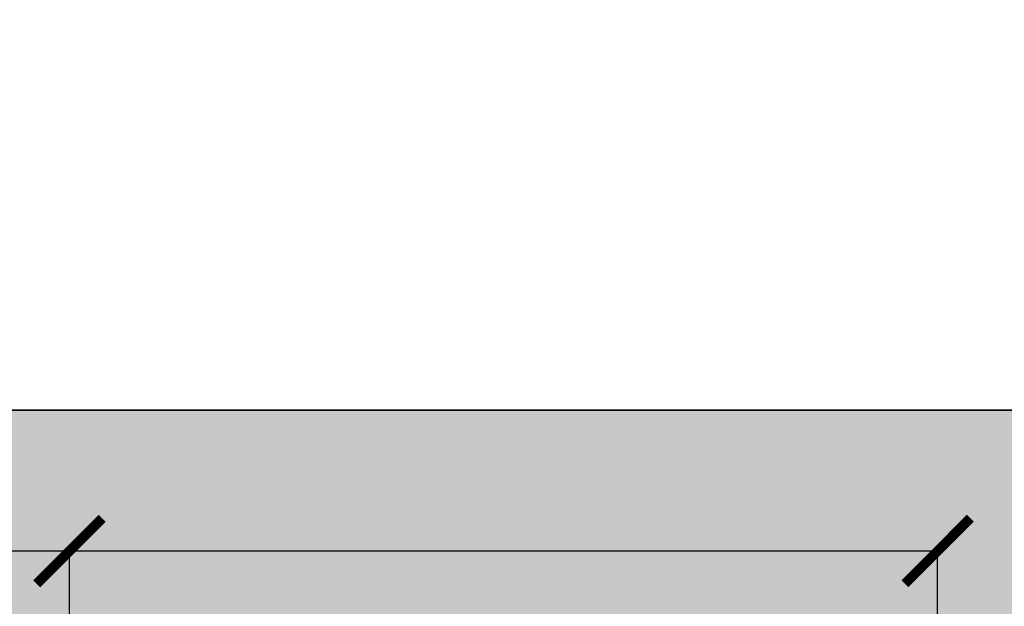
# Model space of a CAD drawing. Units: inches. Extents: x 1704 to 6393, y -157 to 1172.
# Tile 79 of 122: x 2017 to 2048, y 1027 to 1045. Entities that reach past the tile are written whole.
import ezdxf

# ---------------------------------------------------------------- set-up
doc = ezdxf.new("R2010")
doc.units = ezdxf.units.IN
doc.header["$MEASUREMENT"] = 0
doc.layers.add('A-ANNO-DIMS', color=7, linetype='Continuous', lineweight=13)
doc.layers.add('C-PROP', color=7, linetype='Continuous', lineweight=35)
doc.layers.add('L-HRDS-PATT', color=9, linetype='Continuous', lineweight=13, true_color=0xc5c1ba)
doc.styles.get("Standard").update_dxf_attribs({"font": 'arial.ttf'})
doc.dimstyles.get("Standard").update_dxf_attribs({"dimtxt": 6, "dimasz": 2, "dimexe": 0.18, "dimexo": 0.0625, "dimgap": 0.09, "dimtad": 0, "dimtih": 1, "dimtoh": 1, "dimdec": 1, "dimzin": 0, "dimdsep": 46, "dimlunit": 3, "dimtxsty": 'Standard', "dimblk": 'ARCHTICK', "dimcen": 0.09, "dimadec": 0, "dimazin": 0, "dimtfac": 1, "dimtdec": 1, "dimtofl": 0, "dimtmove": 0, "dimatfit": 3, "dimfxl": 1, "dimtolj": 1, "dimtzin": 0, "dimarcsym": 0})

# ---------------------------------------------------------------- blocks, each defined once
blk = doc.blocks.new('_ArchTick')
at = {"color": 0, "linetype": 'ByBlock', "const_width": 0.15}
blk.add_lwpolyline([(-0.5, -0.5), (0.5, 0.5)], dxfattribs=at)
blk = doc.blocks.new('*D80')
at = {"layer": 'A-ANNO-DIMS', "color": 0, "lineweight": -2, "transparency": 16777216}
for p, q in [((2018.966, 1025.001), (2018.966, 1029.096)), ((2045.487, 1025.001), (2045.487, 1029.096)), ((2018.966, 1028.916), (2016.966, 1028.916)), ((2045.487, 1028.916), (2018.966, 1028.916))]:
    blk.add_line(p, q, dxfattribs=at)
at = {"layer": 'Defpoints', "color": 0, "lineweight": -3, "transparency": 16777216}
for p in [(2018.966, 1028.916), (2018.966, 1024.938), (2045.487, 1024.938)]:
    blk.add_point(p, dxfattribs=at)
at = {"layer": 'A-ANNO-DIMS', "color": 0, "lineweight": -2, "transparency": 16777216, "xscale": 2, "yscale": 2, "zscale": 2, "rotation": 180}
blk.add_blockref('_ArchTick', (2018.966, 1028.916), dxfattribs=at)
at = {"layer": 'A-ANNO-DIMS', "color": 0, "lineweight": -2, "transparency": 16777216, "xscale": 2, "yscale": 2, "zscale": 2}
blk.add_blockref('_ArchTick', (2045.487, 1028.916), dxfattribs=at)
at = {"layer": 'A-ANNO-DIMS', "color": 0, "transparency": 16777216, "insert": (1967.173, 1028.916), "char_height": 6, "attachment_point": 5}
blk.add_mtext('\\A1;AUTUMN SHRUB 27 TYP.', dxfattribs=at)
blk = doc.blocks.new('*D94')
at = {"layer": 'A-ANNO-DIMS', "color": 0, "lineweight": -2, "transparency": 16777216}
for p, q in [((1898.349, 895.275), (1898.349, 1105.287)), ((1898.349, 1105.107), (1979.39, 1105.107)), ((2073.349, 1105.107), (1992.307, 1105.107)), ((2073.349, 895.275), (2073.349, 1105.287))]:
    blk.add_line(p, q, dxfattribs=at)
at = {"layer": 'Defpoints', "color": 0, "lineweight": -3, "transparency": 16777216}
for p in [(2073.349, 1105.107), (1898.349, 895.213), (2073.349, 895.213)]:
    blk.add_point(p, dxfattribs=at)
at = {"layer": 'A-ANNO-DIMS', "color": 0, "lineweight": -2, "transparency": 16777216, "xscale": 2, "yscale": 2, "zscale": 2, "rotation": 180}
blk.add_blockref('_ArchTick', (1898.349, 1105.107), dxfattribs=at)
at = {"layer": 'A-ANNO-DIMS', "color": 0, "lineweight": -2, "transparency": 16777216, "xscale": 2, "yscale": 2, "zscale": 2}
blk.add_blockref('_ArchTick', (2073.349, 1105.107), dxfattribs=at)
at = {"layer": 'A-ANNO-DIMS', "color": 0, "transparency": 16777216, "insert": (1985.849, 1105.107), "char_height": 6, "attachment_point": 5}
blk.add_mtext('\\A1;175', dxfattribs=at)

msp = doc.modelspace()

# ---------------------------------------------------------------- hatches: boundary and pattern name
at = {"layer": 'L-HRDS-PATT', "transparency": 33554643}
h = msp.add_hatch(color=256, dxfattribs=at)
h.dxf.hatch_style = 1
h.paths.add_polyline_path([(2065.589, 1033.213), (1898.349, 1033.213), (1898.349, 895.213), (2065.589, 895.213)])

# ---------------------------------------------------------------- linework, layer by layer
at = {"layer": 'C-PROP'}
msp.add_line((2723.349, 1033.213), (1898.349, 1033.213), dxfattribs=at)

# ---------------------------------------------------------------- dimensions: what is measured, and where the dimension line sits
at = {"layer": 'A-ANNO-DIMS'}
dim = msp.add_linear_dim(base=(2073.349, 1105.107), p1=(1898.349, 895.213), p2=(2073.349, 895.213), dimstyle='Standard', override={"dimdec": 0, "dimlfac": 1, "dimrnd": 0, "dimzin": 0, "dimdsep": 46, "dimlunit": 2}, dxfattribs=at)
dim.commit()
dim.dimension.update_dxf_attribs({"geometry": '*D94', "text_midpoint": (1985.849, 1105.107)})
dim = msp.add_linear_dim(base=(2018.966, 1028.916), p1=(2045.487, 1024.938), p2=(2018.966, 1024.938), angle=180, text='AUTUMN SHRUB <> TYP.', dimstyle='Standard', override={"dimdec": 0, "dimlfac": 1, "dimrnd": 0, "dimzin": 0, "dimdsep": 46, "dimlunit": 2}, dxfattribs=at)
dim.commit()
dim.dimension.update_dxf_attribs({"geometry": '*D80', "text_midpoint": (1967.173, 1028.916)})

doc.saveas('drawing.dxf')
